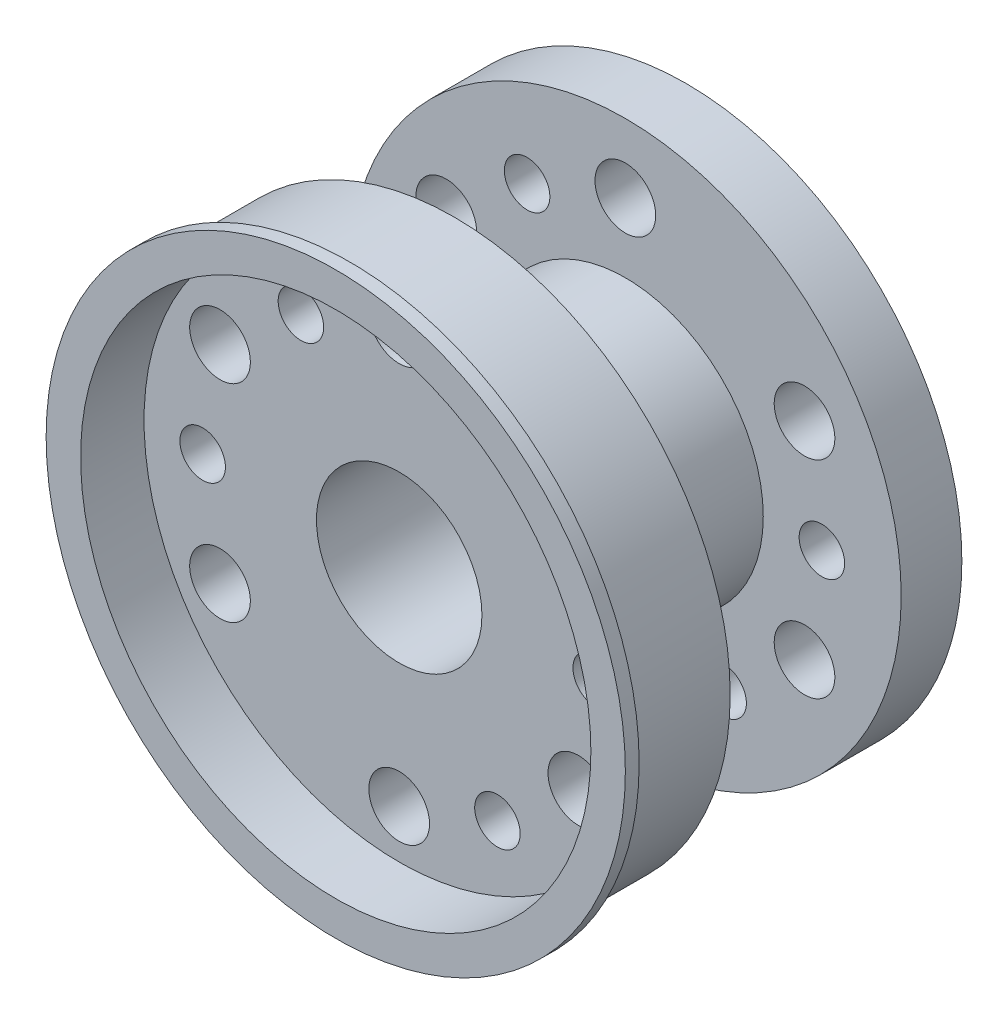
ISO-10303-21;
HEADER;
FILE_DESCRIPTION(('STEP AP214'),'2;1');
FILE_NAME('part.step','',(''),(''),'','','');
FILE_SCHEMA(('AUTOMOTIVE_DESIGN { 1 0 10303 214 1 1 1 1 }'));
ENDSEC;
DATA;
#1=APPLICATION_CONTEXT('core data for automotive mechanical design processes');
#2=APPLICATION_PROTOCOL_DEFINITION('international standard','automotive_design',2000,#1);
#3=PRODUCT_CONTEXT('',#1,'mechanical');
#4=PRODUCT('Part','Part','',(#3));
#5=PRODUCT_RELATED_PRODUCT_CATEGORY('part','',(#4));
#6=PRODUCT_DEFINITION_FORMATION('','',#4);
#7=PRODUCT_DEFINITION_CONTEXT('part definition',#1,'design');
#8=PRODUCT_DEFINITION('design','',#6,#7);
#9=PRODUCT_DEFINITION_SHAPE('','',#8);
#10=(LENGTH_UNIT() NAMED_UNIT(*) SI_UNIT(.MILLI.,.METRE.));
#11=(NAMED_UNIT(*) PLANE_ANGLE_UNIT() SI_UNIT($,.RADIAN.));
#12=(NAMED_UNIT(*) SI_UNIT($,.STERADIAN.) SOLID_ANGLE_UNIT());
#13=UNCERTAINTY_MEASURE_WITH_UNIT(LENGTH_MEASURE(1.E-05),#10,'distance_accuracy_value','');
#14=(GEOMETRIC_REPRESENTATION_CONTEXT(3) GLOBAL_UNCERTAINTY_ASSIGNED_CONTEXT((#13)) GLOBAL_UNIT_ASSIGNED_CONTEXT((#10,
#11,#12)) REPRESENTATION_CONTEXT('',''));
#15=CARTESIAN_POINT('',(0.,0.,0.));
#16=DIRECTION('',(0.,0.,1.));
#17=DIRECTION('',(1.,0.,0.));
#18=AXIS2_PLACEMENT_3D('',#15,#16,#17);
#19=CARTESIAN_POINT('',(0.,0.,-5.));
#20=DIRECTION('',(0.,0.,1.));
#21=DIRECTION('',(1.,0.,0.));
#22=AXIS2_PLACEMENT_3D('',#19,#20,#21);
#23=CYLINDRICAL_SURFACE('',#22,105.);
#24=CARTESIAN_POINT('',(0.,0.,-5.));
#25=DIRECTION('',(0.,0.,1.));
#26=DIRECTION('',(1.,0.,0.));
#27=AXIS2_PLACEMENT_3D('',#24,#25,#26);
#28=CIRCLE('',#27,105.);
#29=CARTESIAN_POINT('',(105.,0.,-5.));
#30=VERTEX_POINT('',#29);
#31=EDGE_CURVE('E47',#30,#30,#28,.T.);
#32=ORIENTED_EDGE('',*,*,#31,.T.);
#33=EDGE_LOOP('',(#32));
#34=FACE_BOUND('',#33,.T.);
#35=CARTESIAN_POINT('',(0.,0.,0.));
#36=DIRECTION('',(0.,0.,1.));
#37=DIRECTION('',(1.,0.,0.));
#38=AXIS2_PLACEMENT_3D('',#35,#36,#37);
#39=CIRCLE('',#38,105.);
#40=CARTESIAN_POINT('',(105.,0.,0.));
#41=VERTEX_POINT('',#40);
#42=EDGE_CURVE('E37',#41,#41,#39,.T.);
#43=ORIENTED_EDGE('',*,*,#42,.F.);
#44=EDGE_LOOP('',(#43));
#45=FACE_BOUND('',#44,.T.);
#46=ADVANCED_FACE('F40',(#34,#45),#23,.T.);
#47=CARTESIAN_POINT('',(0.,0.,-5.));
#48=DIRECTION('',(0.,0.,1.));
#49=DIRECTION('',(1.,0.,0.));
#50=AXIS2_PLACEMENT_3D('',#47,#48,#49);
#51=PLANE('',#50);
#52=CARTESIAN_POINT('',(0.,0.,-5.));
#53=DIRECTION('',(0.,0.,-1.));
#54=DIRECTION('',(-1.,0.,0.));
#55=AXIS2_PLACEMENT_3D('',#52,#53,#54);
#56=CIRCLE('',#55,100.);
#57=CARTESIAN_POINT('',(-100.,0.,-5.));
#58=VERTEX_POINT('',#57);
#59=EDGE_CURVE('E42',#58,#58,#56,.T.);
#60=ORIENTED_EDGE('',*,*,#59,.F.);
#61=EDGE_LOOP('',(#60));
#62=FACE_BOUND('',#61,.T.);
#63=ORIENTED_EDGE('',*,*,#31,.F.);
#64=EDGE_LOOP('',(#63));
#65=FACE_BOUND('',#64,.T.);
#66=ADVANCED_FACE('F66',(#62,#65),#51,.F.);
#67=CARTESIAN_POINT('',(0.,0.,0.));
#68=DIRECTION('',(0.,0.,1.));
#69=DIRECTION('',(1.,0.,0.));
#70=AXIS2_PLACEMENT_3D('',#67,#68,#69);
#71=PLANE('',#70);
#72=CARTESIAN_POINT('',(0.,0.,0.));
#73=DIRECTION('',(0.,0.,1.));
#74=DIRECTION('',(1.,0.,0.));
#75=AXIS2_PLACEMENT_3D('',#72,#73,#74);
#76=CIRCLE('',#75,92.5);
#77=CARTESIAN_POINT('',(92.5,0.,0.));
#78=VERTEX_POINT('',#77);
#79=EDGE_CURVE('E242',#78,#78,#76,.T.);
#80=ORIENTED_EDGE('',*,*,#79,.F.);
#81=EDGE_LOOP('',(#80));
#82=FACE_BOUND('',#81,.T.);
#83=ORIENTED_EDGE('',*,*,#42,.T.);
#84=EDGE_LOOP('',(#83));
#85=FACE_BOUND('',#84,.T.);
#86=ADVANCED_FACE('F61',(#82,#85),#71,.T.);
#87=CARTESIAN_POINT('',(0.,0.,-43.));
#88=DIRECTION('',(0.,0.,1.));
#89=DIRECTION('',(1.,0.,0.));
#90=AXIS2_PLACEMENT_3D('',#87,#88,#89);
#91=CYLINDRICAL_SURFACE('',#90,100.);
#92=CARTESIAN_POINT('',(0.,0.,-43.));
#93=DIRECTION('',(0.,0.,-1.));
#94=DIRECTION('',(-1.,0.,0.));
#95=AXIS2_PLACEMENT_3D('',#92,#93,#94);
#96=CIRCLE('',#95,100.);
#97=CARTESIAN_POINT('',(-100.,0.,-43.));
#98=VERTEX_POINT('',#97);
#99=EDGE_CURVE('E54',#98,#98,#96,.T.);
#100=ORIENTED_EDGE('',*,*,#99,.F.);
#101=EDGE_LOOP('',(#100));
#102=FACE_BOUND('',#101,.T.);
#103=ORIENTED_EDGE('',*,*,#59,.T.);
#104=EDGE_LOOP('',(#103));
#105=FACE_BOUND('',#104,.T.);
#106=ADVANCED_FACE('F78',(#102,#105),#91,.T.);
#107=CARTESIAN_POINT('',(0.,0.,-43.));
#108=DIRECTION('',(0.,0.,-1.));
#109=DIRECTION('',(-1.,0.,0.));
#110=AXIS2_PLACEMENT_3D('',#107,#108,#109);
#111=PLANE('',#110);
#112=CARTESIAN_POINT('',(-35.6250000000001,61.7043100196412,-43.));
#113=DIRECTION('',(0.,0.,-1.));
#114=DIRECTION('',(-1.,0.,0.));
#115=AXIS2_PLACEMENT_3D('',#112,#113,#114);
#116=CIRCLE('',#115,8.24999999999999);
#117=CARTESIAN_POINT('',(-43.8750000000001,61.7043100196412,-43.));
#118=VERTEX_POINT('',#117);
#119=EDGE_CURVE('E236',#118,#118,#116,.T.);
#120=ORIENTED_EDGE('',*,*,#119,.F.);
#121=EDGE_LOOP('',(#120));
#122=FACE_BOUND('',#121,.T.);
#123=CARTESIAN_POINT('',(71.25,0.,-43.));
#124=DIRECTION('',(0.,0.,-1.));
#125=DIRECTION('',(-1.,0.,0.));
#126=AXIS2_PLACEMENT_3D('',#123,#124,#125);
#127=CIRCLE('',#126,8.25);
#128=CARTESIAN_POINT('',(63.,0.,-43.));
#129=VERTEX_POINT('',#128);
#130=EDGE_CURVE('E235',#129,#129,#127,.T.);
#131=ORIENTED_EDGE('',*,*,#130,.F.);
#132=EDGE_LOOP('',(#131));
#133=FACE_BOUND('',#132,.T.);
#134=CARTESIAN_POINT('',(-64.9519052838329,37.5,-43.));
#135=DIRECTION('',(0.,0.,-1.));
#136=DIRECTION('',(-1.,0.,0.));
#137=AXIS2_PLACEMENT_3D('',#134,#135,#136);
#138=CIRCLE('',#137,11.0000000000009);
#139=CARTESIAN_POINT('',(-75.9519052838338,37.5,-43.));
#140=VERTEX_POINT('',#139);
#141=EDGE_CURVE('E228',#140,#140,#138,.T.);
#142=ORIENTED_EDGE('',*,*,#141,.F.);
#143=EDGE_LOOP('',(#142));
#144=FACE_BOUND('',#143,.T.);
#145=CARTESIAN_POINT('',(-64.9519052838329,-37.5,-43.));
#146=DIRECTION('',(0.,0.,-1.));
#147=DIRECTION('',(-1.,0.,0.));
#148=AXIS2_PLACEMENT_3D('',#145,#146,#147);
#149=CIRCLE('',#148,11.0000000000007);
#150=CARTESIAN_POINT('',(-75.9519052838336,-37.5,-43.));
#151=VERTEX_POINT('',#150);
#152=EDGE_CURVE('E219',#151,#151,#149,.T.);
#153=ORIENTED_EDGE('',*,*,#152,.F.);
#154=EDGE_LOOP('',(#153));
#155=FACE_BOUND('',#154,.T.);
#156=CARTESIAN_POINT('',(0.,-75.,-43.));
#157=DIRECTION('',(0.,0.,-1.));
#158=DIRECTION('',(-1.,0.,0.));
#159=AXIS2_PLACEMENT_3D('',#156,#157,#158);
#160=CIRCLE('',#159,11.0000000000005);
#161=CARTESIAN_POINT('',(-11.0000000000005,-75.,-43.));
#162=VERTEX_POINT('',#161);
#163=EDGE_CURVE('E212',#162,#162,#160,.T.);
#164=ORIENTED_EDGE('',*,*,#163,.F.);
#165=EDGE_LOOP('',(#164));
#166=FACE_BOUND('',#165,.T.);
#167=CARTESIAN_POINT('',(64.9519052838329,-37.5,-43.));
#168=DIRECTION('',(0.,0.,-1.));
#169=DIRECTION('',(-1.,0.,0.));
#170=AXIS2_PLACEMENT_3D('',#167,#168,#169);
#171=CIRCLE('',#170,11.0000000000004);
#172=CARTESIAN_POINT('',(53.9519052838326,-37.5,-43.));
#173=VERTEX_POINT('',#172);
#174=EDGE_CURVE('E208',#173,#173,#171,.T.);
#175=ORIENTED_EDGE('',*,*,#174,.F.);
#176=EDGE_LOOP('',(#175));
#177=FACE_BOUND('',#176,.T.);
#178=CARTESIAN_POINT('',(64.9519052838345,37.5,-43.));
#179=DIRECTION('',(0.,0.,-1.));
#180=DIRECTION('',(-1.,0.,0.));
#181=AXIS2_PLACEMENT_3D('',#178,#179,#180);
#182=CIRCLE('',#181,10.999999999999);
#183=CARTESIAN_POINT('',(53.9519052838355,37.5,-43.));
#184=VERTEX_POINT('',#183);
#185=EDGE_CURVE('E205',#184,#184,#182,.T.);
#186=ORIENTED_EDGE('',*,*,#185,.F.);
#187=EDGE_LOOP('',(#186));
#188=FACE_BOUND('',#187,.T.);
#189=CARTESIAN_POINT('',(-71.25,0.,-43.));
#190=DIRECTION('',(0.,0.,-1.));
#191=DIRECTION('',(-1.,0.,0.));
#192=AXIS2_PLACEMENT_3D('',#189,#190,#191);
#193=CIRCLE('',#192,8.25);
#194=CARTESIAN_POINT('',(-79.5,0.,-43.));
#195=VERTEX_POINT('',#194);
#196=EDGE_CURVE('E198',#195,#195,#193,.T.);
#197=ORIENTED_EDGE('',*,*,#196,.F.);
#198=EDGE_LOOP('',(#197));
#199=FACE_BOUND('',#198,.T.);
#200=CARTESIAN_POINT('',(35.6250000000001,-61.7043100196412,-43.));
#201=DIRECTION('',(0.,0.,-1.));
#202=DIRECTION('',(-1.,0.,0.));
#203=AXIS2_PLACEMENT_3D('',#200,#201,#202);
#204=CIRCLE('',#203,8.25);
#205=CARTESIAN_POINT('',(27.3750000000001,-61.7043100196412,-43.));
#206=VERTEX_POINT('',#205);
#207=EDGE_CURVE('E184',#206,#206,#204,.T.);
#208=ORIENTED_EDGE('',*,*,#207,.F.);
#209=EDGE_LOOP('',(#208));
#210=FACE_BOUND('',#209,.T.);
#211=CARTESIAN_POINT('',(0.,75.,-43.));
#212=DIRECTION('',(0.,0.,-1.));
#213=DIRECTION('',(-1.,0.,0.));
#214=AXIS2_PLACEMENT_3D('',#211,#212,#213);
#215=CIRCLE('',#214,11.);
#216=CARTESIAN_POINT('',(-11.,75.,-43.));
#217=VERTEX_POINT('',#216);
#218=EDGE_CURVE('E183',#217,#217,#215,.T.);
#219=ORIENTED_EDGE('',*,*,#218,.F.);
#220=EDGE_LOOP('',(#219));
#221=FACE_BOUND('',#220,.T.);
#222=CARTESIAN_POINT('',(0.,0.,-43.));
#223=DIRECTION('',(0.,0.,-1.));
#224=DIRECTION('',(-1.,0.,0.));
#225=AXIS2_PLACEMENT_3D('',#222,#223,#224);
#226=CIRCLE('',#225,50.);
#227=CARTESIAN_POINT('',(-50.,0.,-43.));
#228=VERTEX_POINT('',#227);
#229=EDGE_CURVE('E10',#228,#228,#226,.T.);
#230=ORIENTED_EDGE('',*,*,#229,.F.);
#231=EDGE_LOOP('',(#230));
#232=FACE_BOUND('',#231,.T.);
#233=ORIENTED_EDGE('',*,*,#99,.T.);
#234=EDGE_LOOP('',(#233));
#235=FACE_BOUND('',#234,.T.);
#236=ADVANCED_FACE('F85',(#122,#133,#144,#155,#166,#177,#188,#199,#210,#221,#232,#235),#111,.T.);
#237=CARTESIAN_POINT('',(0.,0.,-105.));
#238=DIRECTION('',(0.,0.,1.));
#239=DIRECTION('',(1.,0.,0.));
#240=AXIS2_PLACEMENT_3D('',#237,#238,#239);
#241=CYLINDRICAL_SURFACE('',#240,50.);
#242=CARTESIAN_POINT('',(0.,0.,-105.));
#243=DIRECTION('',(0.,0.,-1.));
#244=DIRECTION('',(-1.,0.,0.));
#245=AXIS2_PLACEMENT_3D('',#242,#243,#244);
#246=CIRCLE('',#245,50.);
#247=CARTESIAN_POINT('',(-50.,0.,-105.));
#248=VERTEX_POINT('',#247);
#249=EDGE_CURVE('E52',#248,#248,#246,.T.);
#250=ORIENTED_EDGE('',*,*,#249,.F.);
#251=EDGE_LOOP('',(#250));
#252=FACE_BOUND('',#251,.T.);
#253=ORIENTED_EDGE('',*,*,#229,.T.);
#254=EDGE_LOOP('',(#253));
#255=FACE_BOUND('',#254,.T.);
#256=ADVANCED_FACE('F88',(#252,#255),#241,.T.);
#257=CARTESIAN_POINT('',(0.,0.,-127.));
#258=DIRECTION('',(0.,0.,1.));
#259=DIRECTION('',(1.,0.,0.));
#260=AXIS2_PLACEMENT_3D('',#257,#258,#259);
#261=CYLINDRICAL_SURFACE('',#260,100.);
#262=CARTESIAN_POINT('',(0.,0.,-127.));
#263=DIRECTION('',(0.,0.,-1.));
#264=DIRECTION('',(-1.,0.,0.));
#265=AXIS2_PLACEMENT_3D('',#262,#263,#264);
#266=CIRCLE('',#265,100.);
#267=CARTESIAN_POINT('',(-100.,0.,-127.));
#268=VERTEX_POINT('',#267);
#269=EDGE_CURVE('E255',#268,#268,#266,.T.);
#270=ORIENTED_EDGE('',*,*,#269,.F.);
#271=EDGE_LOOP('',(#270));
#272=FACE_BOUND('',#271,.T.);
#273=CARTESIAN_POINT('',(0.,0.,-105.));
#274=DIRECTION('',(0.,0.,-1.));
#275=DIRECTION('',(-1.,0.,0.));
#276=AXIS2_PLACEMENT_3D('',#273,#274,#275);
#277=CIRCLE('',#276,100.);
#278=CARTESIAN_POINT('',(-100.,0.,-105.));
#279=VERTEX_POINT('',#278);
#280=EDGE_CURVE('E253',#279,#279,#277,.T.);
#281=ORIENTED_EDGE('',*,*,#280,.T.);
#282=EDGE_LOOP('',(#281));
#283=FACE_BOUND('',#282,.T.);
#284=ADVANCED_FACE('F89',(#272,#283),#261,.T.);
#285=CARTESIAN_POINT('',(0.,0.,-127.));
#286=DIRECTION('',(0.,0.,-1.));
#287=DIRECTION('',(-1.,0.,0.));
#288=AXIS2_PLACEMENT_3D('',#285,#286,#287);
#289=PLANE('',#288);
#290=CARTESIAN_POINT('',(-35.6250000000001,61.7043100196412,-127.));
#291=DIRECTION('',(0.,0.,1.));
#292=DIRECTION('',(1.,0.,0.));
#293=AXIS2_PLACEMENT_3D('',#290,#291,#292);
#294=CIRCLE('',#293,8.24999999999999);
#295=CARTESIAN_POINT('',(-27.3750000000001,61.7043100196412,-127.));
#296=VERTEX_POINT('',#295);
#297=EDGE_CURVE('E337',#296,#296,#294,.T.);
#298=ORIENTED_EDGE('',*,*,#297,.T.);
#299=EDGE_LOOP('',(#298));
#300=FACE_BOUND('',#299,.T.);
#301=CARTESIAN_POINT('',(71.25,0.,-127.));
#302=DIRECTION('',(0.,0.,1.));
#303=DIRECTION('',(1.,0.,0.));
#304=AXIS2_PLACEMENT_3D('',#301,#302,#303);
#305=CIRCLE('',#304,8.25);
#306=CARTESIAN_POINT('',(79.5,0.,-127.));
#307=VERTEX_POINT('',#306);
#308=EDGE_CURVE('E347',#307,#307,#305,.T.);
#309=ORIENTED_EDGE('',*,*,#308,.T.);
#310=EDGE_LOOP('',(#309));
#311=FACE_BOUND('',#310,.T.);
#312=CARTESIAN_POINT('',(-64.9519052838329,37.5,-127.));
#313=DIRECTION('',(0.,0.,1.));
#314=DIRECTION('',(1.,0.,0.));
#315=AXIS2_PLACEMENT_3D('',#312,#313,#314);
#316=CIRCLE('',#315,11.0000000000009);
#317=CARTESIAN_POINT('',(-53.951905283832,37.5,-127.));
#318=VERTEX_POINT('',#317);
#319=EDGE_CURVE('E355',#318,#318,#316,.T.);
#320=ORIENTED_EDGE('',*,*,#319,.T.);
#321=EDGE_LOOP('',(#320));
#322=FACE_BOUND('',#321,.T.);
#323=CARTESIAN_POINT('',(-64.9519052838329,-37.5,-127.));
#324=DIRECTION('',(0.,0.,1.));
#325=DIRECTION('',(1.,0.,0.));
#326=AXIS2_PLACEMENT_3D('',#323,#324,#325);
#327=CIRCLE('',#326,11.0000000000007);
#328=CARTESIAN_POINT('',(-53.9519052838322,-37.5,-127.));
#329=VERTEX_POINT('',#328);
#330=EDGE_CURVE('E319',#329,#329,#327,.T.);
#331=ORIENTED_EDGE('',*,*,#330,.T.);
#332=EDGE_LOOP('',(#331));
#333=FACE_BOUND('',#332,.T.);
#334=CARTESIAN_POINT('',(0.,-75.,-127.));
#335=DIRECTION('',(0.,0.,1.));
#336=DIRECTION('',(1.,0.,0.));
#337=AXIS2_PLACEMENT_3D('',#334,#335,#336);
#338=CIRCLE('',#337,11.0000000000005);
#339=CARTESIAN_POINT('',(11.0000000000005,-75.,-127.));
#340=VERTEX_POINT('',#339);
#341=EDGE_CURVE('E317',#340,#340,#338,.T.);
#342=ORIENTED_EDGE('',*,*,#341,.T.);
#343=EDGE_LOOP('',(#342));
#344=FACE_BOUND('',#343,.T.);
#345=CARTESIAN_POINT('',(64.9519052838329,-37.5,-127.));
#346=DIRECTION('',(0.,0.,1.));
#347=DIRECTION('',(1.,0.,0.));
#348=AXIS2_PLACEMENT_3D('',#345,#346,#347);
#349=CIRCLE('',#348,11.0000000000004);
#350=CARTESIAN_POINT('',(75.9519052838333,-37.5,-127.));
#351=VERTEX_POINT('',#350);
#352=EDGE_CURVE('E326',#351,#351,#349,.T.);
#353=ORIENTED_EDGE('',*,*,#352,.T.);
#354=EDGE_LOOP('',(#353));
#355=FACE_BOUND('',#354,.T.);
#356=CARTESIAN_POINT('',(64.9519052838345,37.5,-127.));
#357=DIRECTION('',(0.,0.,1.));
#358=DIRECTION('',(1.,0.,0.));
#359=AXIS2_PLACEMENT_3D('',#356,#357,#358);
#360=CIRCLE('',#359,10.999999999999);
#361=CARTESIAN_POINT('',(75.9519052838335,37.5,-127.));
#362=VERTEX_POINT('',#361);
#363=EDGE_CURVE('E335',#362,#362,#360,.T.);
#364=ORIENTED_EDGE('',*,*,#363,.T.);
#365=EDGE_LOOP('',(#364));
#366=FACE_BOUND('',#365,.T.);
#367=CARTESIAN_POINT('',(-71.25,0.,-127.));
#368=DIRECTION('',(0.,0.,1.));
#369=DIRECTION('',(1.,0.,0.));
#370=AXIS2_PLACEMENT_3D('',#367,#368,#369);
#371=CIRCLE('',#370,8.25);
#372=CARTESIAN_POINT('',(-63.,0.,-127.));
#373=VERTEX_POINT('',#372);
#374=EDGE_CURVE('E303',#373,#373,#371,.T.);
#375=ORIENTED_EDGE('',*,*,#374,.T.);
#376=EDGE_LOOP('',(#375));
#377=FACE_BOUND('',#376,.T.);
#378=CARTESIAN_POINT('',(35.6250000000001,-61.7043100196412,-127.));
#379=DIRECTION('',(0.,0.,1.));
#380=DIRECTION('',(1.,0.,0.));
#381=AXIS2_PLACEMENT_3D('',#378,#379,#380);
#382=CIRCLE('',#381,8.25);
#383=CARTESIAN_POINT('',(43.8750000000001,-61.7043100196412,-127.));
#384=VERTEX_POINT('',#383);
#385=EDGE_CURVE('E178',#384,#384,#382,.T.);
#386=ORIENTED_EDGE('',*,*,#385,.T.);
#387=EDGE_LOOP('',(#386));
#388=FACE_BOUND('',#387,.T.);
#389=CARTESIAN_POINT('',(0.,75.,-127.));
#390=DIRECTION('',(0.,0.,1.));
#391=DIRECTION('',(1.,0.,0.));
#392=AXIS2_PLACEMENT_3D('',#389,#390,#391);
#393=CIRCLE('',#392,11.);
#394=CARTESIAN_POINT('',(11.,75.,-127.));
#395=VERTEX_POINT('',#394);
#396=EDGE_CURVE('E302',#395,#395,#393,.T.);
#397=ORIENTED_EDGE('',*,*,#396,.T.);
#398=EDGE_LOOP('',(#397));
#399=FACE_BOUND('',#398,.T.);
#400=CARTESIAN_POINT('',(0.,0.,-127.));
#401=DIRECTION('',(0.,0.,1.));
#402=DIRECTION('',(1.,0.,0.));
#403=AXIS2_PLACEMENT_3D('',#400,#401,#402);
#404=CIRCLE('',#403,30.);
#405=CARTESIAN_POINT('',(30.,0.,-127.));
#406=VERTEX_POINT('',#405);
#407=EDGE_CURVE('E245',#406,#406,#404,.T.);
#408=ORIENTED_EDGE('',*,*,#407,.T.);
#409=EDGE_LOOP('',(#408));
#410=FACE_BOUND('',#409,.T.);
#411=ORIENTED_EDGE('',*,*,#269,.T.);
#412=EDGE_LOOP('',(#411));
#413=FACE_BOUND('',#412,.T.);
#414=ADVANCED_FACE('F94',(#300,#311,#322,#333,#344,#355,#366,#377,#388,#399,#410,#413),#289,.T.);
#415=CARTESIAN_POINT('',(0.,0.,-105.));
#416=DIRECTION('',(0.,0.,-1.));
#417=DIRECTION('',(-1.,0.,0.));
#418=AXIS2_PLACEMENT_3D('',#415,#416,#417);
#419=PLANE('',#418);
#420=CARTESIAN_POINT('',(-35.6250000000001,61.7043100196412,-105.));
#421=DIRECTION('',(0.,0.,-1.));
#422=DIRECTION('',(-1.,0.,0.));
#423=AXIS2_PLACEMENT_3D('',#420,#421,#422);
#424=CIRCLE('',#423,8.24999999999999);
#425=CARTESIAN_POINT('',(-43.8750000000001,61.7043100196412,-105.));
#426=VERTEX_POINT('',#425);
#427=EDGE_CURVE('E234',#426,#426,#424,.T.);
#428=ORIENTED_EDGE('',*,*,#427,.T.);
#429=EDGE_LOOP('',(#428));
#430=FACE_BOUND('',#429,.T.);
#431=CARTESIAN_POINT('',(71.25,0.,-105.));
#432=DIRECTION('',(0.,0.,-1.));
#433=DIRECTION('',(-1.,0.,0.));
#434=AXIS2_PLACEMENT_3D('',#431,#432,#433);
#435=CIRCLE('',#434,8.25);
#436=CARTESIAN_POINT('',(63.,0.,-105.));
#437=VERTEX_POINT('',#436);
#438=EDGE_CURVE('E229',#437,#437,#435,.T.);
#439=ORIENTED_EDGE('',*,*,#438,.T.);
#440=EDGE_LOOP('',(#439));
#441=FACE_BOUND('',#440,.T.);
#442=CARTESIAN_POINT('',(-64.9519052838329,37.5,-105.));
#443=DIRECTION('',(0.,0.,-1.));
#444=DIRECTION('',(-1.,0.,0.));
#445=AXIS2_PLACEMENT_3D('',#442,#443,#444);
#446=CIRCLE('',#445,11.0000000000009);
#447=CARTESIAN_POINT('',(-75.9519052838338,37.5,-105.));
#448=VERTEX_POINT('',#447);
#449=EDGE_CURVE('E224',#448,#448,#446,.T.);
#450=ORIENTED_EDGE('',*,*,#449,.T.);
#451=EDGE_LOOP('',(#450));
#452=FACE_BOUND('',#451,.T.);
#453=CARTESIAN_POINT('',(-64.9519052838329,-37.5,-105.));
#454=DIRECTION('',(0.,0.,-1.));
#455=DIRECTION('',(-1.,0.,0.));
#456=AXIS2_PLACEMENT_3D('',#453,#454,#455);
#457=CIRCLE('',#456,11.0000000000007);
#458=CARTESIAN_POINT('',(-75.9519052838336,-37.5,-105.));
#459=VERTEX_POINT('',#458);
#460=EDGE_CURVE('E220',#459,#459,#457,.T.);
#461=ORIENTED_EDGE('',*,*,#460,.T.);
#462=EDGE_LOOP('',(#461));
#463=FACE_BOUND('',#462,.T.);
#464=CARTESIAN_POINT('',(0.,-75.,-105.));
#465=DIRECTION('',(0.,0.,-1.));
#466=DIRECTION('',(-1.,0.,0.));
#467=AXIS2_PLACEMENT_3D('',#464,#465,#466);
#468=CIRCLE('',#467,11.0000000000005);
#469=CARTESIAN_POINT('',(-11.0000000000005,-75.,-105.));
#470=VERTEX_POINT('',#469);
#471=EDGE_CURVE('E211',#470,#470,#468,.T.);
#472=ORIENTED_EDGE('',*,*,#471,.T.);
#473=EDGE_LOOP('',(#472));
#474=FACE_BOUND('',#473,.T.);
#475=CARTESIAN_POINT('',(64.9519052838329,-37.5,-105.));
#476=DIRECTION('',(0.,0.,-1.));
#477=DIRECTION('',(-1.,0.,0.));
#478=AXIS2_PLACEMENT_3D('',#475,#476,#477);
#479=CIRCLE('',#478,11.0000000000004);
#480=CARTESIAN_POINT('',(53.9519052838326,-37.5,-105.));
#481=VERTEX_POINT('',#480);
#482=EDGE_CURVE('E202',#481,#481,#479,.T.);
#483=ORIENTED_EDGE('',*,*,#482,.T.);
#484=EDGE_LOOP('',(#483));
#485=FACE_BOUND('',#484,.T.);
#486=CARTESIAN_POINT('',(64.9519052838345,37.5,-105.));
#487=DIRECTION('',(0.,0.,-1.));
#488=DIRECTION('',(-1.,0.,0.));
#489=AXIS2_PLACEMENT_3D('',#486,#487,#488);
#490=CIRCLE('',#489,10.999999999999);
#491=CARTESIAN_POINT('',(53.9519052838355,37.5,-105.));
#492=VERTEX_POINT('',#491);
#493=EDGE_CURVE('E200',#492,#492,#490,.T.);
#494=ORIENTED_EDGE('',*,*,#493,.T.);
#495=EDGE_LOOP('',(#494));
#496=FACE_BOUND('',#495,.T.);
#497=CARTESIAN_POINT('',(-71.25,0.,-105.));
#498=DIRECTION('',(0.,0.,-1.));
#499=DIRECTION('',(-1.,0.,0.));
#500=AXIS2_PLACEMENT_3D('',#497,#498,#499);
#501=CIRCLE('',#500,8.25);
#502=CARTESIAN_POINT('',(-79.5,0.,-105.));
#503=VERTEX_POINT('',#502);
#504=EDGE_CURVE('E190',#503,#503,#501,.T.);
#505=ORIENTED_EDGE('',*,*,#504,.T.);
#506=EDGE_LOOP('',(#505));
#507=FACE_BOUND('',#506,.T.);
#508=CARTESIAN_POINT('',(35.6250000000001,-61.7043100196412,-105.));
#509=DIRECTION('',(0.,0.,-1.));
#510=DIRECTION('',(-1.,0.,0.));
#511=AXIS2_PLACEMENT_3D('',#508,#509,#510);
#512=CIRCLE('',#511,8.25);
#513=CARTESIAN_POINT('',(27.3750000000001,-61.7043100196412,-105.));
#514=VERTEX_POINT('',#513);
#515=EDGE_CURVE('E185',#514,#514,#512,.T.);
#516=ORIENTED_EDGE('',*,*,#515,.T.);
#517=EDGE_LOOP('',(#516));
#518=FACE_BOUND('',#517,.T.);
#519=CARTESIAN_POINT('',(0.,75.,-105.));
#520=DIRECTION('',(0.,0.,-1.));
#521=DIRECTION('',(-1.,0.,0.));
#522=AXIS2_PLACEMENT_3D('',#519,#520,#521);
#523=CIRCLE('',#522,11.);
#524=CARTESIAN_POINT('',(-11.,75.,-105.));
#525=VERTEX_POINT('',#524);
#526=EDGE_CURVE('E187',#525,#525,#523,.T.);
#527=ORIENTED_EDGE('',*,*,#526,.T.);
#528=EDGE_LOOP('',(#527));
#529=FACE_BOUND('',#528,.T.);
#530=ORIENTED_EDGE('',*,*,#249,.T.);
#531=EDGE_LOOP('',(#530));
#532=FACE_BOUND('',#531,.T.);
#533=ORIENTED_EDGE('',*,*,#280,.F.);
#534=EDGE_LOOP('',(#533));
#535=FACE_BOUND('',#534,.T.);
#536=ADVANCED_FACE('F96',(#430,#441,#452,#463,#474,#485,#496,#507,#518,#529,#532,#535),#419,.F.);
#537=CARTESIAN_POINT('',(0.,0.,-23.));
#538=DIRECTION('',(0.,0.,1.));
#539=DIRECTION('',(1.,0.,0.));
#540=AXIS2_PLACEMENT_3D('',#537,#538,#539);
#541=CYLINDRICAL_SURFACE('',#540,92.5);
#542=CARTESIAN_POINT('',(0.,0.,-23.));
#543=DIRECTION('',(0.,0.,1.));
#544=DIRECTION('',(1.,0.,0.));
#545=AXIS2_PLACEMENT_3D('',#542,#543,#544);
#546=CIRCLE('',#545,92.5);
#547=CARTESIAN_POINT('',(92.5,0.,-23.));
#548=VERTEX_POINT('',#547);
#549=EDGE_CURVE('E247',#548,#548,#546,.T.);
#550=ORIENTED_EDGE('',*,*,#549,.F.);
#551=EDGE_LOOP('',(#550));
#552=FACE_BOUND('',#551,.T.);
#553=ORIENTED_EDGE('',*,*,#79,.T.);
#554=EDGE_LOOP('',(#553));
#555=FACE_BOUND('',#554,.T.);
#556=ADVANCED_FACE('F97',(#552,#555),#541,.F.);
#557=CARTESIAN_POINT('',(0.,0.,-23.));
#558=DIRECTION('',(0.,0.,1.));
#559=DIRECTION('',(1.,0.,0.));
#560=AXIS2_PLACEMENT_3D('',#557,#558,#559);
#561=PLANE('',#560);
#562=CARTESIAN_POINT('',(-35.6250000000001,61.7043100196412,-23.));
#563=DIRECTION('',(0.,0.,1.));
#564=DIRECTION('',(1.,0.,0.));
#565=AXIS2_PLACEMENT_3D('',#562,#563,#564);
#566=CIRCLE('',#565,8.24999999999999);
#567=CARTESIAN_POINT('',(-27.3750000000001,61.7043100196412,-23.));
#568=VERTEX_POINT('',#567);
#569=EDGE_CURVE('E340',#568,#568,#566,.T.);
#570=ORIENTED_EDGE('',*,*,#569,.F.);
#571=EDGE_LOOP('',(#570));
#572=FACE_BOUND('',#571,.T.);
#573=CARTESIAN_POINT('',(71.25,0.,-23.));
#574=DIRECTION('',(0.,0.,1.));
#575=DIRECTION('',(1.,0.,0.));
#576=AXIS2_PLACEMENT_3D('',#573,#574,#575);
#577=CIRCLE('',#576,8.25);
#578=CARTESIAN_POINT('',(79.5,0.,-23.));
#579=VERTEX_POINT('',#578);
#580=EDGE_CURVE('E342',#579,#579,#577,.T.);
#581=ORIENTED_EDGE('',*,*,#580,.F.);
#582=EDGE_LOOP('',(#581));
#583=FACE_BOUND('',#582,.T.);
#584=CARTESIAN_POINT('',(-64.9519052838329,37.5,-23.));
#585=DIRECTION('',(0.,0.,1.));
#586=DIRECTION('',(1.,0.,0.));
#587=AXIS2_PLACEMENT_3D('',#584,#585,#586);
#588=CIRCLE('',#587,11.0000000000009);
#589=CARTESIAN_POINT('',(-53.951905283832,37.5,-23.));
#590=VERTEX_POINT('',#589);
#591=EDGE_CURVE('E349',#590,#590,#588,.T.);
#592=ORIENTED_EDGE('',*,*,#591,.F.);
#593=EDGE_LOOP('',(#592));
#594=FACE_BOUND('',#593,.T.);
#595=CARTESIAN_POINT('',(-64.9519052838329,-37.5,-23.));
#596=DIRECTION('',(0.,0.,1.));
#597=DIRECTION('',(1.,0.,0.));
#598=AXIS2_PLACEMENT_3D('',#595,#596,#597);
#599=CIRCLE('',#598,11.0000000000007);
#600=CARTESIAN_POINT('',(-53.9519052838322,-37.5,-23.));
#601=VERTEX_POINT('',#600);
#602=EDGE_CURVE('E352',#601,#601,#599,.T.);
#603=ORIENTED_EDGE('',*,*,#602,.F.);
#604=EDGE_LOOP('',(#603));
#605=FACE_BOUND('',#604,.T.);
#606=CARTESIAN_POINT('',(0.,-75.,-23.));
#607=DIRECTION('',(0.,0.,1.));
#608=DIRECTION('',(1.,0.,0.));
#609=AXIS2_PLACEMENT_3D('',#606,#607,#608);
#610=CIRCLE('',#609,11.0000000000005);
#611=CARTESIAN_POINT('',(11.0000000000005,-75.,-23.));
#612=VERTEX_POINT('',#611);
#613=EDGE_CURVE('E316',#612,#612,#610,.T.);
#614=ORIENTED_EDGE('',*,*,#613,.F.);
#615=EDGE_LOOP('',(#614));
#616=FACE_BOUND('',#615,.T.);
#617=CARTESIAN_POINT('',(64.9519052838329,-37.5,-23.));
#618=DIRECTION('',(0.,0.,1.));
#619=DIRECTION('',(1.,0.,0.));
#620=AXIS2_PLACEMENT_3D('',#617,#618,#619);
#621=CIRCLE('',#620,11.0000000000004);
#622=CARTESIAN_POINT('',(75.9519052838333,-37.5,-23.));
#623=VERTEX_POINT('',#622);
#624=EDGE_CURVE('E323',#623,#623,#621,.T.);
#625=ORIENTED_EDGE('',*,*,#624,.F.);
#626=EDGE_LOOP('',(#625));
#627=FACE_BOUND('',#626,.T.);
#628=CARTESIAN_POINT('',(64.9519052838345,37.5,-23.));
#629=DIRECTION('',(0.,0.,1.));
#630=DIRECTION('',(1.,0.,0.));
#631=AXIS2_PLACEMENT_3D('',#628,#629,#630);
#632=CIRCLE('',#631,10.999999999999);
#633=CARTESIAN_POINT('',(75.9519052838335,37.5,-23.));
#634=VERTEX_POINT('',#633);
#635=EDGE_CURVE('E328',#634,#634,#632,.T.);
#636=ORIENTED_EDGE('',*,*,#635,.F.);
#637=EDGE_LOOP('',(#636));
#638=FACE_BOUND('',#637,.T.);
#639=CARTESIAN_POINT('',(-71.25,0.,-23.));
#640=DIRECTION('',(0.,0.,1.));
#641=DIRECTION('',(1.,0.,0.));
#642=AXIS2_PLACEMENT_3D('',#639,#640,#641);
#643=CIRCLE('',#642,8.25);
#644=CARTESIAN_POINT('',(-63.,0.,-23.));
#645=VERTEX_POINT('',#644);
#646=EDGE_CURVE('E310',#645,#645,#643,.T.);
#647=ORIENTED_EDGE('',*,*,#646,.F.);
#648=EDGE_LOOP('',(#647));
#649=FACE_BOUND('',#648,.T.);
#650=CARTESIAN_POINT('',(35.6250000000001,-61.7043100196412,-23.));
#651=DIRECTION('',(0.,0.,1.));
#652=DIRECTION('',(1.,0.,0.));
#653=AXIS2_PLACEMENT_3D('',#650,#651,#652);
#654=CIRCLE('',#653,8.25);
#655=CARTESIAN_POINT('',(43.8750000000001,-61.7043100196412,-23.));
#656=VERTEX_POINT('',#655);
#657=EDGE_CURVE('E359',#656,#656,#654,.T.);
#658=ORIENTED_EDGE('',*,*,#657,.F.);
#659=EDGE_LOOP('',(#658));
#660=FACE_BOUND('',#659,.T.);
#661=CARTESIAN_POINT('',(0.,75.,-23.));
#662=DIRECTION('',(0.,0.,1.));
#663=DIRECTION('',(1.,0.,0.));
#664=AXIS2_PLACEMENT_3D('',#661,#662,#663);
#665=CIRCLE('',#664,11.);
#666=CARTESIAN_POINT('',(11.,75.,-23.));
#667=VERTEX_POINT('',#666);
#668=EDGE_CURVE('E301',#667,#667,#665,.T.);
#669=ORIENTED_EDGE('',*,*,#668,.F.);
#670=EDGE_LOOP('',(#669));
#671=FACE_BOUND('',#670,.T.);
#672=CARTESIAN_POINT('',(0.,0.,-23.));
#673=DIRECTION('',(0.,0.,1.));
#674=DIRECTION('',(1.,0.,0.));
#675=AXIS2_PLACEMENT_3D('',#672,#673,#674);
#676=CIRCLE('',#675,30.);
#677=CARTESIAN_POINT('',(30.,0.,-23.));
#678=VERTEX_POINT('',#677);
#679=EDGE_CURVE('E243',#678,#678,#676,.T.);
#680=ORIENTED_EDGE('',*,*,#679,.F.);
#681=EDGE_LOOP('',(#680));
#682=FACE_BOUND('',#681,.T.);
#683=ORIENTED_EDGE('',*,*,#549,.T.);
#684=EDGE_LOOP('',(#683));
#685=FACE_BOUND('',#684,.T.);
#686=ADVANCED_FACE('F106',(#572,#583,#594,#605,#616,#627,#638,#649,#660,#671,#682,#685),#561,.T.);
#687=CARTESIAN_POINT('',(0.,0.,-127.));
#688=DIRECTION('',(0.,0.,1.));
#689=DIRECTION('',(1.,0.,0.));
#690=AXIS2_PLACEMENT_3D('',#687,#688,#689);
#691=CYLINDRICAL_SURFACE('',#690,30.);
#692=ORIENTED_EDGE('',*,*,#407,.F.);
#693=EDGE_LOOP('',(#692));
#694=FACE_BOUND('',#693,.T.);
#695=ORIENTED_EDGE('',*,*,#679,.T.);
#696=EDGE_LOOP('',(#695));
#697=FACE_BOUND('',#696,.T.);
#698=ADVANCED_FACE('F109',(#694,#697),#691,.F.);
#699=CARTESIAN_POINT('',(0.,75.,-127.));
#700=DIRECTION('',(0.,0.,1.));
#701=DIRECTION('',(1.,0.,0.));
#702=AXIS2_PLACEMENT_3D('',#699,#700,#701);
#703=CYLINDRICAL_SURFACE('',#702,11.);
#704=ORIENTED_EDGE('',*,*,#218,.T.);
#705=EDGE_LOOP('',(#704));
#706=FACE_BOUND('',#705,.T.);
#707=ORIENTED_EDGE('',*,*,#668,.T.);
#708=EDGE_LOOP('',(#707));
#709=FACE_BOUND('',#708,.T.);
#710=ADVANCED_FACE('F111',(#706,#709),#703,.F.);
#711=CARTESIAN_POINT('',(35.6250000000001,-61.7043100196412,-127.));
#712=DIRECTION('',(0.,0.,1.));
#713=DIRECTION('',(1.,0.,0.));
#714=AXIS2_PLACEMENT_3D('',#711,#712,#713);
#715=CYLINDRICAL_SURFACE('',#714,8.25);
#716=ORIENTED_EDGE('',*,*,#207,.T.);
#717=EDGE_LOOP('',(#716));
#718=FACE_BOUND('',#717,.T.);
#719=ORIENTED_EDGE('',*,*,#657,.T.);
#720=EDGE_LOOP('',(#719));
#721=FACE_BOUND('',#720,.T.);
#722=ADVANCED_FACE('F116',(#718,#721),#715,.F.);
#723=CARTESIAN_POINT('',(-71.25,0.,-127.));
#724=DIRECTION('',(0.,0.,1.));
#725=DIRECTION('',(1.,0.,0.));
#726=AXIS2_PLACEMENT_3D('',#723,#724,#725);
#727=CYLINDRICAL_SURFACE('',#726,8.25);
#728=ORIENTED_EDGE('',*,*,#196,.T.);
#729=EDGE_LOOP('',(#728));
#730=FACE_BOUND('',#729,.T.);
#731=ORIENTED_EDGE('',*,*,#646,.T.);
#732=EDGE_LOOP('',(#731));
#733=FACE_BOUND('',#732,.T.);
#734=ADVANCED_FACE('F132',(#730,#733),#727,.F.);
#735=CARTESIAN_POINT('',(64.9519052838345,37.5,-127.));
#736=DIRECTION('',(0.,0.,1.));
#737=DIRECTION('',(1.,0.,0.));
#738=AXIS2_PLACEMENT_3D('',#735,#736,#737);
#739=CYLINDRICAL_SURFACE('',#738,10.999999999999);
#740=ORIENTED_EDGE('',*,*,#185,.T.);
#741=EDGE_LOOP('',(#740));
#742=FACE_BOUND('',#741,.T.);
#743=ORIENTED_EDGE('',*,*,#635,.T.);
#744=EDGE_LOOP('',(#743));
#745=FACE_BOUND('',#744,.T.);
#746=ADVANCED_FACE('F128',(#742,#745),#739,.F.);
#747=CARTESIAN_POINT('',(64.9519052838329,-37.5,-127.));
#748=DIRECTION('',(0.,0.,1.));
#749=DIRECTION('',(1.,0.,0.));
#750=AXIS2_PLACEMENT_3D('',#747,#748,#749);
#751=CYLINDRICAL_SURFACE('',#750,11.0000000000004);
#752=ORIENTED_EDGE('',*,*,#174,.T.);
#753=EDGE_LOOP('',(#752));
#754=FACE_BOUND('',#753,.T.);
#755=ORIENTED_EDGE('',*,*,#624,.T.);
#756=EDGE_LOOP('',(#755));
#757=FACE_BOUND('',#756,.T.);
#758=ADVANCED_FACE('F124',(#754,#757),#751,.F.);
#759=CARTESIAN_POINT('',(0.,-75.,-127.));
#760=DIRECTION('',(0.,0.,1.));
#761=DIRECTION('',(1.,0.,0.));
#762=AXIS2_PLACEMENT_3D('',#759,#760,#761);
#763=CYLINDRICAL_SURFACE('',#762,11.0000000000005);
#764=ORIENTED_EDGE('',*,*,#163,.T.);
#765=EDGE_LOOP('',(#764));
#766=FACE_BOUND('',#765,.T.);
#767=ORIENTED_EDGE('',*,*,#613,.T.);
#768=EDGE_LOOP('',(#767));
#769=FACE_BOUND('',#768,.T.);
#770=ADVANCED_FACE('F121',(#766,#769),#763,.F.);
#771=CARTESIAN_POINT('',(-64.9519052838329,-37.5,-127.));
#772=DIRECTION('',(0.,0.,1.));
#773=DIRECTION('',(1.,0.,0.));
#774=AXIS2_PLACEMENT_3D('',#771,#772,#773);
#775=CYLINDRICAL_SURFACE('',#774,11.0000000000007);
#776=ORIENTED_EDGE('',*,*,#152,.T.);
#777=EDGE_LOOP('',(#776));
#778=FACE_BOUND('',#777,.T.);
#779=ORIENTED_EDGE('',*,*,#602,.T.);
#780=EDGE_LOOP('',(#779));
#781=FACE_BOUND('',#780,.T.);
#782=ADVANCED_FACE('F123',(#778,#781),#775,.F.);
#783=CARTESIAN_POINT('',(-64.9519052838329,37.5,-127.));
#784=DIRECTION('',(0.,0.,1.));
#785=DIRECTION('',(1.,0.,0.));
#786=AXIS2_PLACEMENT_3D('',#783,#784,#785);
#787=CYLINDRICAL_SURFACE('',#786,11.0000000000009);
#788=ORIENTED_EDGE('',*,*,#141,.T.);
#789=EDGE_LOOP('',(#788));
#790=FACE_BOUND('',#789,.T.);
#791=ORIENTED_EDGE('',*,*,#591,.T.);
#792=EDGE_LOOP('',(#791));
#793=FACE_BOUND('',#792,.T.);
#794=ADVANCED_FACE('F147',(#790,#793),#787,.F.);
#795=CARTESIAN_POINT('',(71.25,0.,-127.));
#796=DIRECTION('',(0.,0.,1.));
#797=DIRECTION('',(1.,0.,0.));
#798=AXIS2_PLACEMENT_3D('',#795,#796,#797);
#799=CYLINDRICAL_SURFACE('',#798,8.25);
#800=ORIENTED_EDGE('',*,*,#130,.T.);
#801=EDGE_LOOP('',(#800));
#802=FACE_BOUND('',#801,.T.);
#803=ORIENTED_EDGE('',*,*,#580,.T.);
#804=EDGE_LOOP('',(#803));
#805=FACE_BOUND('',#804,.T.);
#806=ADVANCED_FACE('F144',(#802,#805),#799,.F.);
#807=CARTESIAN_POINT('',(-35.6250000000001,61.7043100196412,-127.));
#808=DIRECTION('',(0.,0.,1.));
#809=DIRECTION('',(1.,0.,0.));
#810=AXIS2_PLACEMENT_3D('',#807,#808,#809);
#811=CYLINDRICAL_SURFACE('',#810,8.24999999999999);
#812=ORIENTED_EDGE('',*,*,#119,.T.);
#813=EDGE_LOOP('',(#812));
#814=FACE_BOUND('',#813,.T.);
#815=ORIENTED_EDGE('',*,*,#569,.T.);
#816=EDGE_LOOP('',(#815));
#817=FACE_BOUND('',#816,.T.);
#818=ADVANCED_FACE('F142',(#814,#817),#811,.F.);
#819=ORIENTED_EDGE('',*,*,#396,.F.);
#820=EDGE_LOOP('',(#819));
#821=FACE_BOUND('',#820,.T.);
#822=ORIENTED_EDGE('',*,*,#526,.F.);
#823=EDGE_LOOP('',(#822));
#824=FACE_BOUND('',#823,.T.);
#825=ADVANCED_FACE('F117',(#821,#824),#703,.F.);
#826=ORIENTED_EDGE('',*,*,#385,.F.);
#827=EDGE_LOOP('',(#826));
#828=FACE_BOUND('',#827,.T.);
#829=ORIENTED_EDGE('',*,*,#515,.F.);
#830=EDGE_LOOP('',(#829));
#831=FACE_BOUND('',#830,.T.);
#832=ADVANCED_FACE('F162',(#828,#831),#715,.F.);
#833=ORIENTED_EDGE('',*,*,#374,.F.);
#834=EDGE_LOOP('',(#833));
#835=FACE_BOUND('',#834,.T.);
#836=ORIENTED_EDGE('',*,*,#504,.F.);
#837=EDGE_LOOP('',(#836));
#838=FACE_BOUND('',#837,.T.);
#839=ADVANCED_FACE('F143',(#835,#838),#727,.F.);
#840=ORIENTED_EDGE('',*,*,#363,.F.);
#841=EDGE_LOOP('',(#840));
#842=FACE_BOUND('',#841,.T.);
#843=ORIENTED_EDGE('',*,*,#493,.F.);
#844=EDGE_LOOP('',(#843));
#845=FACE_BOUND('',#844,.T.);
#846=ADVANCED_FACE('F140',(#842,#845),#739,.F.);
#847=ORIENTED_EDGE('',*,*,#352,.F.);
#848=EDGE_LOOP('',(#847));
#849=FACE_BOUND('',#848,.T.);
#850=ORIENTED_EDGE('',*,*,#482,.F.);
#851=EDGE_LOOP('',(#850));
#852=FACE_BOUND('',#851,.T.);
#853=ADVANCED_FACE('F135',(#849,#852),#751,.F.);
#854=ORIENTED_EDGE('',*,*,#341,.F.);
#855=EDGE_LOOP('',(#854));
#856=FACE_BOUND('',#855,.T.);
#857=ORIENTED_EDGE('',*,*,#471,.F.);
#858=EDGE_LOOP('',(#857));
#859=FACE_BOUND('',#858,.T.);
#860=ADVANCED_FACE('F130',(#856,#859),#763,.F.);
#861=ORIENTED_EDGE('',*,*,#330,.F.);
#862=EDGE_LOOP('',(#861));
#863=FACE_BOUND('',#862,.T.);
#864=ORIENTED_EDGE('',*,*,#460,.F.);
#865=EDGE_LOOP('',(#864));
#866=FACE_BOUND('',#865,.T.);
#867=ADVANCED_FACE('F159',(#863,#866),#775,.F.);
#868=ORIENTED_EDGE('',*,*,#319,.F.);
#869=EDGE_LOOP('',(#868));
#870=FACE_BOUND('',#869,.T.);
#871=ORIENTED_EDGE('',*,*,#449,.F.);
#872=EDGE_LOOP('',(#871));
#873=FACE_BOUND('',#872,.T.);
#874=ADVANCED_FACE('F156',(#870,#873),#787,.F.);
#875=ORIENTED_EDGE('',*,*,#308,.F.);
#876=EDGE_LOOP('',(#875));
#877=FACE_BOUND('',#876,.T.);
#878=ORIENTED_EDGE('',*,*,#438,.F.);
#879=EDGE_LOOP('',(#878));
#880=FACE_BOUND('',#879,.T.);
#881=ADVANCED_FACE('F155',(#877,#880),#799,.F.);
#882=ORIENTED_EDGE('',*,*,#297,.F.);
#883=EDGE_LOOP('',(#882));
#884=FACE_BOUND('',#883,.T.);
#885=ORIENTED_EDGE('',*,*,#427,.F.);
#886=EDGE_LOOP('',(#885));
#887=FACE_BOUND('',#886,.T.);
#888=ADVANCED_FACE('F150',(#884,#887),#811,.F.);
#889=CLOSED_SHELL('',(#46,#66,#86,#106,#236,#256,#284,#414,#536,#556,#686,#698,#710,#722,#734,
#746,#758,#770,#782,#794,#806,#818,#825,#832,#839,#846,#853,#860,#867,#874,#881,#888));
#890=MANIFOLD_SOLID_BREP('B2',#889);
#891=ADVANCED_BREP_SHAPE_REPRESENTATION('',(#18,#890),#14);
#892=SHAPE_DEFINITION_REPRESENTATION(#9,#891);
ENDSEC;
END-ISO-10303-21;
